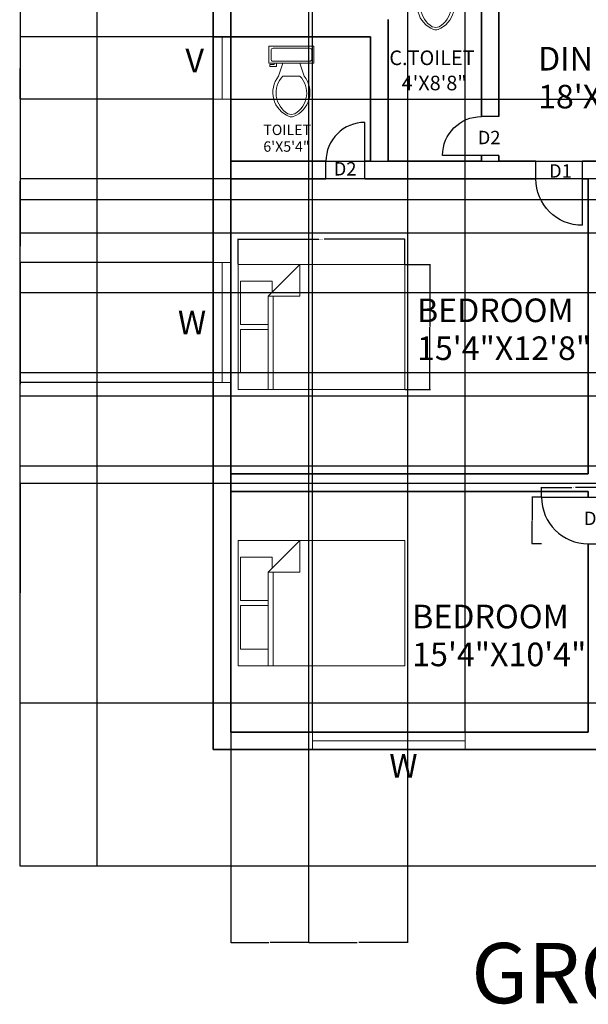
# Model space of a CAD drawing. Units: feet. Extents: x 2270 to 3094, y 1543 to 2352.
# Tile 1 of 6: x 2270 to 2563, y 1543 to 2050. Entities that reach past the tile are written whole.
import ezdxf

# ---------------------------------------------------------------- set-up
doc = ezdxf.new("R2010")
doc.units = ezdxf.units.FT
for name, color, linetype, lineweight in [('A-ANNO-DIMS', 2, 'Continuous', 18), ('A-ANNO-TEXT', 7, 'Continuous', 18), ('A-ANNO-TITL', 7, 'Continuous', 35), ('A-AREA-IDEN', 7, 'Continuous', 18), ('A-DOOR', 3, 'Continuous', 25), ('A-FLOR-FIXT', 8, 'Continuous', 18), ('A-FURN', 8, 'Continuous', 18), ('A-GLAZ', 4, 'Continuous', 18), ('A-WALL', 7, 'Continuous', 35), ('C-PROP', 8, 'Continuous', 25)]:
    doc.layers.add(name, color=color, linetype=linetype, lineweight=lineweight)
doc.styles.get("Standard").update_dxf_attribs({"font": 'arial.ttf'})
doc.dimstyles.get("Standard").update_dxf_attribs({"dimtxt": 0.18, "dimasz": 0.18, "dimexe": 0.18, "dimexo": 0.0625, "dimgap": 0.09, "dimtad": 0, "dimtih": 1, "dimtoh": 1, "dimdec": 4, "dimzin": 0, "dimdsep": 46, "dimtxsty": 'Standard', "dimcen": 0.09, "dimadec": 0, "dimazin": 0, "dimtfac": 1, "dimtdec": 4, "dimtofl": 0, "dimtmove": 0, "dimatfit": 3, "dimfxl": 1, "dimtolj": 1, "dimtzin": 0, "dimarcsym": 0})

# ---------------------------------------------------------------- blocks, each defined once
blk = doc.blocks.new('Toilet - top')
for p, q in [((9.5, -6), (9.5, -2)), ((-10, -8.5), (-8, -8.5)), ((-10, -9.5), (-10, -8.5)), ((-8, -8.5), (-8, -8)), ((-7, -8), (-7, -9.5)), ((-4, -8), (-6, -14)), ((4, -8), (6, -14)), ((-7, -9.5), (-10, -9.5)), ((4, -14), (-4, -14))]:
    blk.add_line(p, q)
blk.add_lwpolyline([(10.5, -8), (10.5, 0), (-10.5, 0), (-10.5, -8)], close=True)
for points in [[(-9.5, -2), (-9.5, -6)], [(8.5, -1), (-8.5, -1)], [(-8.5, -7), (8.5, -7)]]:
    blk.add_lwpolyline(points)
for centre, radius, start, end in [((-8.62, -1.88), 0.884, 81.8699, 188.1301), ((8.62, -1.88), 0.884, 351.8699, 98.1301), ((-8.62, -6.12), 0.884, 171.8699, 278.1301), ((8.62, -6.12), 0.884, 261.8699, 8.1301), ((3.52, -21.58), 12.17, 141.4691, 247.9714), ((4.2, -21.82), 11.33, 136.3677, 238.9468), ((-3.52, -21.58), 12.17, 292.0284, 38.5307), ((-4.2, -21.82), 11.33, 301.053, 43.6321), ((0, -27.88), 4, 245.7318, 294.2682), ((0, -29), 4, 254.8605, 285.1395)]:
    blk.add_arc(centre, radius, start, end)
blk = doc.blocks.new('Bed - Queen')
for p, q in [((0, -80.00003), (0, 0)), ((0, 0), (59.99999, 0)), ((59.99999, 0), (59.99999, -80.00003)), ((7.99999, -1.2), (28.79998, -1.2)), ((7.99999, -14.4), (7.99999, -1.2)), ((28.79998, -1.2), (28.79998, -14.4)), ((31.19999, -1.2), (51.99999, -1.2)), ((31.19999, -14.4), (31.19999, -1.2)), ((51.99999, -1.2), (51.99999, -16.4)), ((0, -14.4), (44.8, -14.4)), ((44.8, -16.8), (0, -16.8)), ((59.99999, -29.6), (44.8, -14.4)), ((44.8, -14.4), (44.8, -29.6)), ((51.99999, -16.4), (46.79936, -16.4)), ((44.8, -29.6), (59.99999, -29.6)), ((59.99999, -80.00003), (0, -80.00003))]:
    blk.add_line(p, q)
blk = doc.blocks.new('DOOR-SWING-24')
blk.add_line((33, 0), (0, 0))
blk.add_arc((9, 0), 24, 0, 90)
blk = doc.blocks.new('DOOR-SWING-20')
blk.add_line((0, 0), (29, 0))
blk.add_arc((9, 0), 20, 0, 90)
blk = doc.blocks.new('*D10')
at = {"layer": 'A-ANNO-DIMS', "color": 0, "lineweight": -2, "transparency": 16777216}
for p, q in [((2538.67, 1804.15), (2538.67, 1809.21)), ((2538.85, 1809.03), (2554.23, 1809.03)), ((2571.49, 1809.03), (2556.1, 1809.03)), ((2571.67, 1804.15), (2571.67, 1809.21))]:
    blk.add_line(p, q, dxfattribs=at)
at = {"layer": 'A-ANNO-DIMS', "color": 0, "transparency": 16777216}
for points in [[(2538.85, 1809.06), (2538.85, 1809), (2538.67, 1809.03)], [(2571.49, 1809.06), (2571.49, 1809), (2571.67, 1809.03)]]:
    blk.add_solid(points, dxfattribs=at)
at = {"layer": 'Defpoints', "color": 0, "transparency": 16777216}
for p in [(2538.67, 1809.03), (2538.67, 1804.08), (2571.67, 1804.08)]:
    blk.add_point(p, dxfattribs=at)
at = {"layer": 'A-ANNO-DIMS', "color": 0, "transparency": 16777216, "insert": (2555.17, 1809.03), "char_height": 0.18, "attachment_point": 5}
blk.add_mtext('\\A1;DOOR 33 TYP.', dxfattribs=at)
blk = doc.blocks.new('*D11')
at = {"layer": 'A-ANNO-DIMS', "color": 0, "lineweight": -2, "transparency": 16777216}
for p, q in [((2538.6, 1804.08), (2533.54, 1804.08)), ((2533.72, 1803.9), (2533.72, 1792.26)), ((2533.72, 1780.26), (2533.72, 1791.9)), ((2538.6, 1780.08), (2533.54, 1780.08))]:
    blk.add_line(p, q, dxfattribs=at)
at = {"layer": 'A-ANNO-DIMS', "color": 0, "transparency": 16777216}
for points in [[(2533.69, 1803.9), (2533.75, 1803.9), (2533.72, 1804.08)], [(2533.69, 1780.26), (2533.75, 1780.26), (2533.72, 1780.08)]]:
    blk.add_solid(points, dxfattribs=at)
at = {"layer": 'Defpoints', "color": 0, "transparency": 16777216}
for p in [(2538.67, 1804.08), (2533.72, 1780.08), (2538.67, 1780.08)]:
    blk.add_point(p, dxfattribs=at)
at = {"layer": 'A-ANNO-DIMS', "color": 0, "transparency": 16777216, "insert": (2533.72, 1792.08), "char_height": 0.18, "attachment_point": 5}
blk.add_mtext('\\A1;24 TYP.', dxfattribs=at)
blk = doc.blocks.new('*D16')
at = {"layer": 'A-ANNO-DIMS', "color": 0, "lineweight": -2, "transparency": 16777216}
for p, q in [((2382.4, 1924.06), (2382.4, 1937.06)), ((2382.58, 1936.88), (2424.06, 1936.88)), ((2468.14, 1936.88), (2426.66, 1936.88)), ((2468.32, 1924.06), (2468.32, 1937.06))]:
    blk.add_line(p, q, dxfattribs=at)
at = {"layer": 'A-ANNO-DIMS', "color": 0, "transparency": 16777216}
for points in [[(2382.58, 1936.91), (2382.58, 1936.85), (2382.4, 1936.88)], [(2468.14, 1936.91), (2468.14, 1936.85), (2468.32, 1936.88)]]:
    blk.add_solid(points, dxfattribs=at)
at = {"layer": 'Defpoints', "color": 0, "transparency": 16777216}
for p in [(2382.4, 1936.88), (2382.4, 1923.99), (2468.32, 1923.99)]:
    blk.add_point(p, dxfattribs=at)
at = {"layer": 'A-ANNO-DIMS', "color": 0, "transparency": 16777216, "insert": (2425.36, 1936.88), "char_height": 0.18, "attachment_point": 5}
blk.add_mtext('\\A1;QUEEN BED 86 TYP.', dxfattribs=at)
blk = doc.blocks.new('*D17')
at = {"layer": 'A-ANNO-DIMS', "color": 0, "lineweight": -2, "transparency": 16777216}
for p, q in [((2468.38, 1923.99), (2481.38, 1923.99)), ((2481.2, 1923.81), (2481.2, 1891.96)), ((2481.2, 1859.74), (2481.2, 1891.59)), ((2468.38, 1859.56), (2481.38, 1859.56))]:
    blk.add_line(p, q, dxfattribs=at)
at = {"layer": 'A-ANNO-DIMS', "color": 0, "transparency": 16777216}
for points in [[(2481.17, 1923.81), (2481.23, 1923.81), (2481.2, 1923.99)], [(2481.17, 1859.74), (2481.23, 1859.74), (2481.2, 1859.56)]]:
    blk.add_solid(points, dxfattribs=at)
at = {"layer": 'Defpoints', "color": 0, "transparency": 16777216}
for p in [(2468.32, 1923.99), (2481.2, 1923.99), (2468.32, 1859.56)]:
    blk.add_point(p, dxfattribs=at)
at = {"layer": 'A-ANNO-DIMS', "color": 0, "transparency": 16777216, "insert": (2481.2, 1891.78), "char_height": 0.18, "attachment_point": 5}
blk.add_mtext('\\A1;64 TYP.', dxfattribs=at)
blk = doc.blocks.new('*D27')
at = {"layer": 'A-ANNO-DIMS', "color": 0, "lineweight": -2, "transparency": 16777216}
for p, q in [((2309.6, 2312.08), (2270.19, 2312.08)), ((2270.37, 2311.9), (2270.37, 1963.27)), ((2270.37, 1614.26), (2270.37, 1962.9)), ((2309.6, 1614.08), (2270.19, 1614.08))]:
    blk.add_line(p, q, dxfattribs=at)
at = {"layer": 'A-ANNO-DIMS', "color": 0, "transparency": 16777216}
for points in [[(2270.34, 2311.9), (2270.4, 2311.9), (2270.37, 2312.08)], [(2270.34, 1614.26), (2270.4, 1614.26), (2270.37, 1614.08)]]:
    blk.add_solid(points, dxfattribs=at)
at = {"layer": 'Defpoints', "color": 0, "transparency": 16777216}
for p in [(2270.37, 2312.08), (2309.67, 2312.08), (2309.67, 1614.08)]:
    blk.add_point(p, dxfattribs=at)
at = {"layer": 'A-ANNO-DIMS', "color": 0, "transparency": 16777216, "insert": (2270.37, 1963.08), "char_height": 0.18, "attachment_point": 5}
blk.add_mtext('\\A1;698', dxfattribs=at)
blk = doc.blocks.new('*D32')
at = {"layer": 'A-ANNO-DIMS', "color": 0, "lineweight": -2, "transparency": 16777216}
for p, q in [((2378.67, 2243.02), (2378.67, 1574.6)), ((2418.6, 2243.02), (2418.6, 1574.6)), ((2378.85, 1574.78), (2398.24, 1574.78)), ((2418.42, 1574.78), (2399.02, 1574.78))]:
    blk.add_line(p, q, dxfattribs=at)
at = {"layer": 'A-ANNO-DIMS', "color": 0, "transparency": 16777216}
for points in [[(2378.85, 1574.81), (2378.85, 1574.75), (2378.67, 1574.78)], [(2418.42, 1574.81), (2418.42, 1574.75), (2418.6, 1574.78)]]:
    blk.add_solid(points, dxfattribs=at)
at = {"layer": 'Defpoints', "color": 0, "transparency": 16777216}
for p in [(2378.67, 2243.08), (2418.6, 2243.08), (2418.6, 1574.78)]:
    blk.add_point(p, dxfattribs=at)
at = {"layer": 'A-ANNO-DIMS', "color": 0, "transparency": 16777216, "insert": (2398.63, 1574.78), "char_height": 0.18, "attachment_point": 5}
blk.add_mtext('\\A1;39.93', dxfattribs=at)
blk = doc.blocks.new('*D33')
at = {"layer": 'A-ANNO-DIMS', "color": 0, "lineweight": -2, "transparency": 16777216}
for p, q in [((2418.6, 2243.02), (2418.6, 1574.6)), ((2469.65, 2243.02), (2469.65, 1574.6)), ((2418.78, 1574.78), (2443.73, 1574.78)), ((2469.47, 1574.78), (2444.52, 1574.78))]:
    blk.add_line(p, q, dxfattribs=at)
at = {"layer": 'A-ANNO-DIMS', "color": 0, "transparency": 16777216}
for points in [[(2418.78, 1574.81), (2418.78, 1574.75), (2418.6, 1574.78)], [(2469.47, 1574.81), (2469.47, 1574.75), (2469.65, 1574.78)]]:
    blk.add_solid(points, dxfattribs=at)
at = {"layer": 'Defpoints', "color": 0, "transparency": 16777216}
for p in [(2418.6, 2243.08), (2469.65, 2243.08), (2469.65, 1574.78)]:
    blk.add_point(p, dxfattribs=at)
at = {"layer": 'A-ANNO-DIMS', "color": 0, "transparency": 16777216, "insert": (2444.12, 1574.78), "char_height": 0.18, "attachment_point": 5}
blk.add_mtext('\\A1;51.05', dxfattribs=at)
blk = doc.blocks.new('*D44')
at = {"layer": 'A-ANNO-DIMS', "color": 0, "lineweight": -2, "transparency": 16777216}
for p, q in [((2816.6, 1957.26), (2270.19, 1957.26)), ((2270.37, 1957.08), (2270.37, 1933.44)), ((2270.37, 1909.44), (2270.37, 1933.08)), ((2816.6, 1909.26), (2270.19, 1909.26))]:
    blk.add_line(p, q, dxfattribs=at)
at = {"layer": 'A-ANNO-DIMS', "color": 0, "transparency": 16777216}
for points in [[(2270.34, 1957.08), (2270.4, 1957.08), (2270.37, 1957.26)], [(2270.34, 1909.44), (2270.4, 1909.44), (2270.37, 1909.26)]]:
    blk.add_solid(points, dxfattribs=at)
at = {"layer": 'Defpoints', "color": 0, "transparency": 16777216}
for p in [(2270.37, 1957.26), (2816.67, 1957.26), (2816.67, 1909.26)]:
    blk.add_point(p, dxfattribs=at)
at = {"layer": 'A-ANNO-DIMS', "color": 0, "transparency": 16777216, "insert": (2270.37, 1933.26), "char_height": 0.18, "attachment_point": 5}
blk.add_mtext('\\A1;48', dxfattribs=at)
blk = doc.blocks.new('*D45')
at = {"layer": 'A-ANNO-DIMS', "color": 0, "lineweight": -2, "transparency": 16777216}
for p, q in [((2816.6, 1909.26), (2270.19, 1909.26)), ((2270.37, 1909.08), (2270.37, 1864.85)), ((2270.37, 1820.26), (2270.37, 1864.49)), ((2816.6, 1820.08), (2270.19, 1820.08))]:
    blk.add_line(p, q, dxfattribs=at)
at = {"layer": 'A-ANNO-DIMS', "color": 0, "transparency": 16777216}
for points in [[(2270.34, 1909.08), (2270.4, 1909.08), (2270.37, 1909.26)], [(2270.34, 1820.26), (2270.4, 1820.26), (2270.37, 1820.08)]]:
    blk.add_solid(points, dxfattribs=at)
at = {"layer": 'Defpoints', "color": 0, "transparency": 16777216}
for p in [(2270.37, 1909.26), (2816.67, 1909.26), (2816.67, 1820.08)]:
    blk.add_point(p, dxfattribs=at)
at = {"layer": 'A-ANNO-DIMS', "color": 0, "transparency": 16777216, "insert": (2270.37, 1864.67), "char_height": 0.18, "attachment_point": 5}
blk.add_mtext('\\A1;89.18', dxfattribs=at)
blk = doc.blocks.new('*D49')
at = {"layer": 'A-ANNO-DIMS', "color": 0, "lineweight": -2, "transparency": 16777216}
for p, q in [((2801.6, 1811.08), (2270.19, 1811.08)), ((2270.37, 1810.9), (2270.37, 1754.77)), ((2270.37, 1698.26), (2270.37, 1754.4)), ((2801.6, 1698.08), (2270.19, 1698.08))]:
    blk.add_line(p, q, dxfattribs=at)
at = {"layer": 'A-ANNO-DIMS', "color": 0, "transparency": 16777216}
for points in [[(2270.34, 1810.9), (2270.4, 1810.9), (2270.37, 1811.08)], [(2270.34, 1698.26), (2270.4, 1698.26), (2270.37, 1698.08)]]:
    blk.add_solid(points, dxfattribs=at)
at = {"layer": 'Defpoints', "color": 0, "transparency": 16777216}
for p in [(2270.37, 1811.08), (2801.67, 1811.08), (2801.67, 1698.08)]:
    blk.add_point(p, dxfattribs=at)
at = {"layer": 'A-ANNO-DIMS', "color": 0, "transparency": 16777216, "insert": (2270.37, 1754.58), "char_height": 0.18, "attachment_point": 5}
blk.add_mtext('\\A1;113', dxfattribs=at)
blk = doc.blocks.new('*D50')
at = {"layer": 'A-ANNO-DIMS', "color": 0, "lineweight": -2, "transparency": 16777216}
for p, q in [((2378.67, 1683.15), (2378.67, 2351.56)), ((2378.85, 2351.38), (2399.3, 2351.38)), ((2420.55, 2351.38), (2400.1, 2351.38)), ((2420.73, 1683.15), (2420.73, 2351.56))]:
    blk.add_line(p, q, dxfattribs=at)
at = {"layer": 'A-ANNO-DIMS', "color": 0, "transparency": 16777216}
for points in [[(2378.85, 2351.41), (2378.85, 2351.35), (2378.67, 2351.38)], [(2420.55, 2351.41), (2420.55, 2351.35), (2420.73, 2351.38)]]:
    blk.add_solid(points, dxfattribs=at)
at = {"layer": 'Defpoints', "color": 0, "transparency": 16777216}
for p in [(2420.73, 2351.38), (2378.67, 1683.08), (2420.73, 1683.08)]:
    blk.add_point(p, dxfattribs=at)
at = {"layer": 'A-ANNO-DIMS', "color": 0, "transparency": 16777216, "insert": (2399.7, 2351.38), "char_height": 0.18, "attachment_point": 5}
blk.add_mtext('\\A1;42.07', dxfattribs=at)
blk = doc.blocks.new('*D51')
at = {"layer": 'A-ANNO-DIMS', "color": 0, "lineweight": -2, "transparency": 16777216}
for p, q in [((2420.73, 1683.15), (2420.73, 2351.56)), ((2420.91, 2351.38), (2459.61, 2351.38)), ((2499.1, 2351.38), (2460.4, 2351.38)), ((2499.28, 1683.15), (2499.28, 2351.56))]:
    blk.add_line(p, q, dxfattribs=at)
at = {"layer": 'A-ANNO-DIMS', "color": 0, "transparency": 16777216}
for points in [[(2420.91, 2351.41), (2420.91, 2351.35), (2420.73, 2351.38)], [(2499.1, 2351.41), (2499.1, 2351.35), (2499.28, 2351.38)]]:
    blk.add_solid(points, dxfattribs=at)
at = {"layer": 'Defpoints', "color": 0, "transparency": 16777216}
for p in [(2499.28, 2351.38), (2420.73, 1683.08), (2499.28, 1683.08)]:
    blk.add_point(p, dxfattribs=at)
at = {"layer": 'A-ANNO-DIMS', "color": 0, "transparency": 16777216, "insert": (2460.01, 2351.38), "char_height": 0.18, "attachment_point": 5}
blk.add_mtext('\\A1;78.55', dxfattribs=at)
blk = doc.blocks.new('*D54')
at = {"layer": 'A-ANNO-DIMS', "color": 0, "lineweight": -2, "transparency": 16777216}
for p, q in [((2369.6, 2009.08), (2270.19, 2009.08)), ((2270.37, 2008.9), (2270.37, 1967.17)), ((2270.37, 1925.06), (2270.37, 1966.8)), ((2369.6, 1924.88), (2270.19, 1924.88))]:
    blk.add_line(p, q, dxfattribs=at)
at = {"layer": 'A-ANNO-DIMS', "color": 0, "transparency": 16777216}
for points in [[(2270.34, 2008.9), (2270.4, 2008.9), (2270.37, 2009.08)], [(2270.34, 1925.06), (2270.4, 1925.06), (2270.37, 1924.88)]]:
    blk.add_solid(points, dxfattribs=at)
at = {"layer": 'Defpoints', "color": 0, "transparency": 16777216}
for p in [(2270.37, 2009.08), (2369.67, 2009.08), (2369.67, 1924.88)]:
    blk.add_point(p, dxfattribs=at)
at = {"layer": 'A-ANNO-DIMS', "color": 0, "transparency": 16777216, "insert": (2270.37, 1966.98), "char_height": 0.18, "attachment_point": 5}
blk.add_mtext('\\A1;84.2', dxfattribs=at)
blk = doc.blocks.new('*D55')
at = {"layer": 'A-ANNO-DIMS', "color": 0, "lineweight": -2, "transparency": 16777216}
for p, q in [((2369.6, 1924.88), (2270.19, 1924.88)), ((2270.37, 1924.7), (2270.37, 1894.2)), ((2270.37, 1863.34), (2270.37, 1893.84)), ((2369.6, 1863.16), (2270.19, 1863.16))]:
    blk.add_line(p, q, dxfattribs=at)
at = {"layer": 'A-ANNO-DIMS', "color": 0, "transparency": 16777216}
for points in [[(2270.34, 1924.7), (2270.4, 1924.7), (2270.37, 1924.88)], [(2270.34, 1863.34), (2270.4, 1863.34), (2270.37, 1863.16)]]:
    blk.add_solid(points, dxfattribs=at)
at = {"layer": 'Defpoints', "color": 0, "transparency": 16777216}
for p in [(2270.37, 1924.88), (2369.67, 1924.88), (2369.67, 1863.16)]:
    blk.add_point(p, dxfattribs=at)
at = {"layer": 'A-ANNO-DIMS', "color": 0, "transparency": 16777216, "insert": (2270.37, 1894.02), "char_height": 0.18, "attachment_point": 5}
blk.add_mtext('\\A1;61.73', dxfattribs=at)
blk = doc.blocks.new('*D56')
at = {"layer": 'A-ANNO-DIMS', "color": 0, "lineweight": -2, "transparency": 16777216}
for p, q in [((2378.73, 2009.08), (3094.15, 2009.08)), ((3093.97, 2008.9), (3093.97, 1993.27)), ((3093.97, 1977.26), (3093.97, 1992.9)), ((2378.73, 1977.08), (3094.15, 1977.08))]:
    blk.add_line(p, q, dxfattribs=at)
at = {"layer": 'A-ANNO-DIMS', "color": 0, "transparency": 16777216}
for points in [[(3093.94, 2008.9), (3094, 2008.9), (3093.97, 2009.08)], [(3093.94, 1977.26), (3094, 1977.26), (3093.97, 1977.08)]]:
    blk.add_solid(points, dxfattribs=at)
at = {"layer": 'Defpoints', "color": 0, "transparency": 16777216}
for p in [(2378.67, 2009.08), (3093.97, 2009.08), (2378.67, 1977.08)]:
    blk.add_point(p, dxfattribs=at)
at = {"layer": 'A-ANNO-DIMS', "color": 0, "transparency": 16777216, "insert": (3093.97, 1993.08), "char_height": 0.18, "attachment_point": 5}
blk.add_mtext('\\A1;32', dxfattribs=at)
blk = doc.blocks.new('*D57')
at = {"layer": 'A-ANNO-DIMS', "color": 0, "lineweight": -2, "transparency": 16777216}
for p, q in [((2369.6, 2041.08), (2270.19, 2041.08)), ((2270.37, 2040.9), (2270.37, 2025.27)), ((2270.37, 2009.26), (2270.37, 2024.9)), ((2369.6, 2009.08), (2270.19, 2009.08))]:
    blk.add_line(p, q, dxfattribs=at)
at = {"layer": 'A-ANNO-DIMS', "color": 0, "transparency": 16777216}
for points in [[(2270.34, 2040.9), (2270.4, 2040.9), (2270.37, 2041.08)], [(2270.34, 2009.26), (2270.4, 2009.26), (2270.37, 2009.08)]]:
    blk.add_solid(points, dxfattribs=at)
at = {"layer": 'Defpoints', "color": 0, "transparency": 16777216}
for p in [(2270.37, 2041.08), (2369.67, 2041.08), (2369.67, 2009.08)]:
    blk.add_point(p, dxfattribs=at)
at = {"layer": 'A-ANNO-DIMS', "color": 0, "transparency": 16777216, "insert": (2270.37, 2025.08), "char_height": 0.18, "attachment_point": 5}
blk.add_mtext('\\A1;32', dxfattribs=at)
blk = doc.blocks.new('*D62')
at = {"layer": 'A-ANNO-DIMS', "color": 0, "lineweight": -2, "transparency": 16777216}
for p, q in [((2571.6, 1868.08), (2270.19, 1868.08)), ((2270.37, 1867.9), (2270.37, 1862.26)), ((2270.37, 1856.26), (2270.37, 1861.9)), ((2571.6, 1856.08), (2270.19, 1856.08))]:
    blk.add_line(p, q, dxfattribs=at)
at = {"layer": 'A-ANNO-DIMS', "color": 0, "transparency": 16777216}
for points in [[(2270.34, 1867.9), (2270.4, 1867.9), (2270.37, 1868.08)], [(2270.34, 1856.26), (2270.4, 1856.26), (2270.37, 1856.08)]]:
    blk.add_solid(points, dxfattribs=at)
at = {"layer": 'Defpoints', "color": 0, "transparency": 16777216}
for p in [(2270.37, 1868.08), (2571.67, 1868.08), (2571.67, 1856.08)]:
    blk.add_point(p, dxfattribs=at)
at = {"layer": 'A-ANNO-DIMS', "color": 0, "transparency": 16777216, "insert": (2270.37, 1862.08), "char_height": 0.18, "attachment_point": 5}
blk.add_mtext('\\A1;12', dxfattribs=at)
blk = doc.blocks.new('*D63')
at = {"layer": 'A-ANNO-DIMS', "color": 0, "lineweight": -2, "transparency": 16777216}
for p, q in [((2655.6, 1968.08), (2270.19, 1968.08)), ((2270.37, 1967.9), (2270.37, 1954.27)), ((2270.37, 1940.26), (2270.37, 1953.9)), ((2655.6, 1940.08), (2270.19, 1940.08))]:
    blk.add_line(p, q, dxfattribs=at)
at = {"layer": 'A-ANNO-DIMS', "color": 0, "transparency": 16777216}
for points in [[(2270.34, 1967.9), (2270.4, 1967.9), (2270.37, 1968.08)], [(2270.34, 1940.26), (2270.4, 1940.26), (2270.37, 1940.08)]]:
    blk.add_solid(points, dxfattribs=at)
at = {"layer": 'Defpoints', "color": 0, "transparency": 16777216}
for p in [(2270.37, 1968.08), (2655.67, 1968.08), (2655.67, 1940.08)]:
    blk.add_point(p, dxfattribs=at)
at = {"layer": 'A-ANNO-DIMS', "color": 0, "transparency": 16777216, "insert": (2270.37, 1954.08), "char_height": 0.18, "attachment_point": 5}
blk.add_mtext('\\A1;28', dxfattribs=at)

msp = doc.modelspace()

# ---------------------------------------------------------------- linework, layer by layer
at = {"layer": 'A-DOOR'}
for p, q in [((2516.6659, 2000.0845), (2507.6659, 2000.0845)), ((2427.6659, 1968.0845), (2427.6659, 1977.0845)), ((2535.6659, 1968.0845), (2535.6659, 1977.0845)), ((2562.6659, 1780.0845), (2571.6659, 1780.0845))]:
    msp.add_line(p, q, dxfattribs=at)
at = {"layer": 'A-GLAZ'}
for p, q in [((2374.1659, 2009.0845), (2374.1659, 2041.0845)), ((2369.6659, 2009.0845), (2378.6659, 2009.0845)), ((2369.6659, 1924.8836), (2378.6659, 1924.8836)), ((2374.1659, 1924.8836), (2374.1659, 1863.1561)), ((2369.6659, 1863.1561), (2378.6659, 1863.1561)), ((2420.7322, 1683.0845), (2420.7322, 1674.0845)), ((2420.7322, 1678.5845), (2499.2818, 1678.5845)), ((2499.2818, 1683.0845), (2499.2818, 1674.0845))]:
    msp.add_line(p, q, dxfattribs=at)
at = {"layer": 'A-WALL'}
for p, q in [((2369.6659, 2098.0845), (2369.6659, 1674.0845)), ((2507.6659, 2086.0845), (2507.6659, 2000.0845)), ((2516.6659, 2086.0845), (2516.6659, 2000.0845)), ((2459.6659, 1977.0845), (2459.6659, 2050.0845)), ((2369.6659, 2041.0845), (2450.6659, 2041.0845)), ((2369.6659, 2041.0845), (2369.6659, 1977.0845)), ((2378.6659, 2041.0845), (2378.6659, 1977.0845)), ((2450.6659, 1977.0845), (2450.6659, 2041.0845)), ((2507.6659, 1980.0845), (2507.6659, 1977.0845)), ((2516.6659, 1980.0845), (2516.6659, 1977.0845)), ((2378.6659, 1977.0845), (2427.6659, 1977.0845)), ((2447.6659, 1977.0845), (2450.6659, 1977.0845)), ((2459.6659, 1977.0845), (2507.6659, 1977.0845)), ((2507.6659, 1977.0845), (2483.6659, 1977.0845)), ((2516.6659, 1977.0845), (2535.6659, 1977.0845)), ((2535.6659, 1977.0845), (2516.6659, 1977.0845)), ((2562.6659, 1977.0845), (2559.6659, 1977.0845)), ((2559.6659, 1977.0845), (2574.6659, 1977.0845)), ((2378.6659, 1968.0845), (2427.6659, 1968.0845)), ((2378.6659, 1968.0845), (2427.6659, 1968.0845)), ((2378.6659, 1968.0845), (2378.6659, 1816.0845)), ((2447.6659, 1968.0845), (2450.6659, 1968.0845)), ((2447.6659, 1968.0845), (2507.6659, 1968.0845)), ((2535.6659, 1968.0845), (2483.6659, 1968.0845)), ((2562.6659, 1968.0845), (2559.6659, 1968.0845)), ((2562.6659, 1816.0845), (2562.6659, 1968.0845)), ((2378.6659, 1816.0845), (2562.6659, 1816.0845)), ((2369.6659, 1807.0845), (2369.6659, 1674.0845)), ((2378.6659, 1807.0845), (2562.6659, 1807.0845)), ((2378.6659, 1807.0845), (2378.6659, 1683.0845)), ((2562.6659, 1804.0845), (2562.6659, 1807.0845)), ((2562.6659, 1683.0845), (2562.6659, 1780.0845)), ((2378.6659, 1683.0845), (2562.6659, 1683.0845)), ((2369.6659, 1674.0845), (2664.6659, 1674.0845))]:
    msp.add_line(p, q, dxfattribs=at)
at = {"layer": 'C-PROP'}
for p in [(2309.6659, 2312.0845), (3054.6659, 1614.0845)]:
    msp.add_line(p, (2309.6659, 1614.0845), dxfattribs=at)

# ---------------------------------------------------------------- block references
at = {"layer": 'A-DOOR', "extrusion": (0, 0, -1), "zscale": -1}
msp.add_blockref('DOOR-SWING-20', (-2516.6658, 1980.085), dxfattribs=at)
at = {"layer": 'A-DOOR'}
for name, p, rotation in [('DOOR-SWING-20', (2447.6654, 1968.0846), 89.9999999999993), ('DOOR-SWING-24', (2571.6658, 1804.084), 180)]:
    msp.add_blockref(name, p, dxfattribs=dict(at, rotation=rotation))
at = {"layer": 'A-DOOR', "extrusion": (0, 0, -1), "zscale": -1, "rotation": 269.9999999999989}
msp.add_blockref('DOOR-SWING-24', (-2559.6654, 1977.0844), dxfattribs=at)
at = {"layer": 'A-FLOR-FIXT', "xscale": 1.103431246609896, "yscale": 1.103431246609896, "zscale": 1.103431246609896}
for p in [(2484.1878, 2081.1448), (2409.8728, 2036.3405)]:
    msp.add_blockref('Toilet - top', p, dxfattribs=at)
at = {"layer": 'A-FURN', "xscale": 1.073910050689623, "yscale": 1.073910050689623, "zscale": 1.073910050689623, "rotation": 90}
for p in [(2382.4037, 1859.5584), (2382.4037, 1717.3018)]:
    msp.add_blockref('Bed - Queen', p, dxfattribs=at)

# ---------------------------------------------------------------- texts
at = {"layer": 'A-ANNO-TEXT'}
for s, height, p in [('V', 12.1456, (2355.346, 2022.8613)), ('D2', 6.89564, (2505.7746, 1985.8574)), ('D2', 6.89564, (2431.6741, 1969.7317)), ('D1', 6.89564, (2542.4675, 1968.6541)), ('W', 12.1456, (2351.4604, 1888.0261)), ('D1', 6.89564, (2560.4382, 1789.7406)), ('W', 12.1456, (2460.2551, 1659.6895))]:
    msp.add_text(s, height=height, dxfattribs=at).set_placement(p)
at = {"layer": 'A-ANNO-TITL'}
msp.add_text('GROUND FLOOR', height=31.058177, dxfattribs=at).set_placement((2502.4393, 1543.4965))
at = {"layer": 'A-AREA-IDEN'}
for s, height, p in [('C.TOILET', 7.51904, (2460.2741, 2026.6)), ('DINING', 12.14556, (2536.8128, 2023.7996)), ('4\'X8\'8"', 7.51904, (2466.6203, 2013.6155)), ('18\'X8\'8"', 12.14556, (2536.8128, 2004.2888)), ('TOILET', 5.34774, (2395.4318, 1990.5755)), ('6\'X5\'4"', 5.34774, (2395.4318, 1981.9848)), ('BEDROOM', 12.14556, (2474.5268, 1894.2467)), ('15\'4"X12\'8"', 12.145557, (2474.5268, 1874.7359)), ('BEDROOM', 12.14556, (2472.0436, 1736.5656)), ('15\'4"X10\'4"', 12.145557, (2472.0436, 1717.0548))]:
    msp.add_text(s, height=height, dxfattribs=at).set_placement(p)

# ---------------------------------------------------------------- dimensions: what is measured, and where the dimension line sits
at = {"layer": 'A-ANNO-DIMS'}
for base, p1, p2, picture, middle in [((2420.7322, 2351.3845), (2378.6659, 1683.0845), (2420.7322, 1683.0845), '*D50', (2399.6991, 2351.3845)), ((2499.2818, 2351.3845), (2420.7322, 1683.0845), (2499.2818, 1683.0845), '*D51', (2460.007, 2351.3845)), ((2418.5967, 1574.7845), (2378.6659, 2243.0845), (2418.5967, 2243.0845), '*D32', (2398.6313, 1574.7845)), ((2469.6502, 1574.7845), (2418.5967, 2243.0845), (2469.6502, 2243.0845), '*D33', (2444.1234, 1574.7845))]:
    dim = msp.add_linear_dim(base=base, p1=p1, p2=p2, dimstyle='Standard', override={"dimdec": 2, "dimlfac": 1, "dimrnd": 0, "dimzin": 0, "dimdsep": 46, "dimlunit": 2}, dxfattribs=at)
    dim.commit()
    dim.dimension.update_dxf_attribs({"geometry": picture, "text_midpoint": middle})
for base, p1, p2, override, picture, middle in [((2270.3659, 2312.0845), (2309.6659, 1614.0845), (2309.6659, 2312.0845), {"dimdec": 0, "dimlfac": 1, "dimrnd": 0, "dimzin": 0, "dimdsep": 46, "dimlunit": 2}, '*D27', (2270.3659, 1963.0845)), ((2270.3659, 2041.0845), (2369.6659, 2009.0845), (2369.6659, 2041.0845), {"dimdec": 0, "dimlfac": 1, "dimrnd": 0, "dimzin": 0, "dimdsep": 46, "dimlunit": 2}, '*D57', (2270.3659, 2025.0845)), ((2270.3659, 2009.0845), (2369.6659, 1924.8836), (2369.6659, 2009.0845), {"dimdec": 1, "dimlfac": 1, "dimrnd": 0, "dimzin": 0, "dimdsep": 46, "dimlunit": 2}, '*D54', (2270.3659, 1966.984)), ((3093.9659, 2009.0845), (2378.6659, 1977.0845), (2378.6659, 2009.0845), {"dimdec": 0, "dimlfac": 1, "dimrnd": 0, "dimzin": 0, "dimdsep": 46, "dimlunit": 2}, '*D56', (3093.9659, 1993.0845)), ((2270.3659, 1968.0845), (2655.6659, 1940.0845), (2655.6659, 1968.0845), {"dimdec": 0, "dimlfac": 1, "dimrnd": 0, "dimzin": 0, "dimdsep": 46, "dimlunit": 2}, '*D63', (2270.3659, 1954.0845)), ((2270.3659, 1957.2599), (2816.6659, 1909.2599), (2816.6659, 1957.2599), {"dimdec": 0, "dimlfac": 1, "dimrnd": 0, "dimzin": 0, "dimdsep": 46, "dimlunit": 2}, '*D44', (2270.3659, 1933.2599)), ((2270.3659, 1924.8836), (2369.6659, 1863.1561), (2369.6659, 1924.8836), {"dimdec": 2, "dimlfac": 1, "dimrnd": 0, "dimzin": 0, "dimdsep": 46, "dimlunit": 2}, '*D55', (2270.3659, 1894.0199)), ((2270.3659, 1909.2599), (2816.6659, 1820.0845), (2816.6659, 1909.2599), {"dimdec": 2, "dimlfac": 1, "dimrnd": 0, "dimzin": 0, "dimdsep": 46, "dimlunit": 2}, '*D45', (2270.3659, 1864.6722)), ((2270.3659, 1868.0845), (2571.6659, 1856.0845), (2571.6659, 1868.0845), {"dimdec": 0, "dimlfac": 1, "dimrnd": 0, "dimzin": 0, "dimdsep": 46, "dimlunit": 2}, '*D62', (2270.3659, 1862.0845)), ((2270.3659, 1811.0845), (2801.6659, 1698.0845), (2801.6659, 1811.0845), {"dimdec": 0, "dimlfac": 1, "dimrnd": 0, "dimzin": 0, "dimdsep": 46, "dimlunit": 2}, '*D49', (2270.3659, 1754.5845))]:
    dim = msp.add_linear_dim(base=base, p1=p1, p2=p2, angle=90, dimstyle='Standard', override=override, dxfattribs=at)
    dim.commit()
    dim.dimension.update_dxf_attribs({"geometry": picture, "text_midpoint": middle})
for base, p1, p2, angle, text, picture, middle in [((2382.4037, 1936.8799), (2468.3165, 1923.993), (2382.4037, 1923.993), 180, 'QUEEN BED <> TYP.', '*D16', (2425.3601, 1936.8799)), ((2481.2034, 1923.993), (2468.3165, 1859.5584), (2468.3165, 1923.993), 90, '<> TYP.', '*D17', (2481.2034, 1891.7757)), ((2538.6659, 1809.0345), (2571.6659, 1804.0845), (2538.6659, 1804.0845), 180, 'DOOR <> TYP.', '*D10', (2555.1659, 1809.0345)), ((2533.7159, 1780.0845), (2538.6659, 1804.0845), (2538.6659, 1780.0845), 270, '<> TYP.', '*D11', (2533.7159, 1792.0845))]:
    dim = msp.add_linear_dim(base=base, p1=p1, p2=p2, angle=angle, text=text, dimstyle='Standard', override={"dimdec": 0, "dimlfac": 1, "dimrnd": 0, "dimzin": 0, "dimdsep": 46, "dimlunit": 2}, dxfattribs=at)
    dim.commit()
    dim.dimension.update_dxf_attribs({"geometry": picture, "text_midpoint": middle})

doc.saveas('drawing.dxf')
